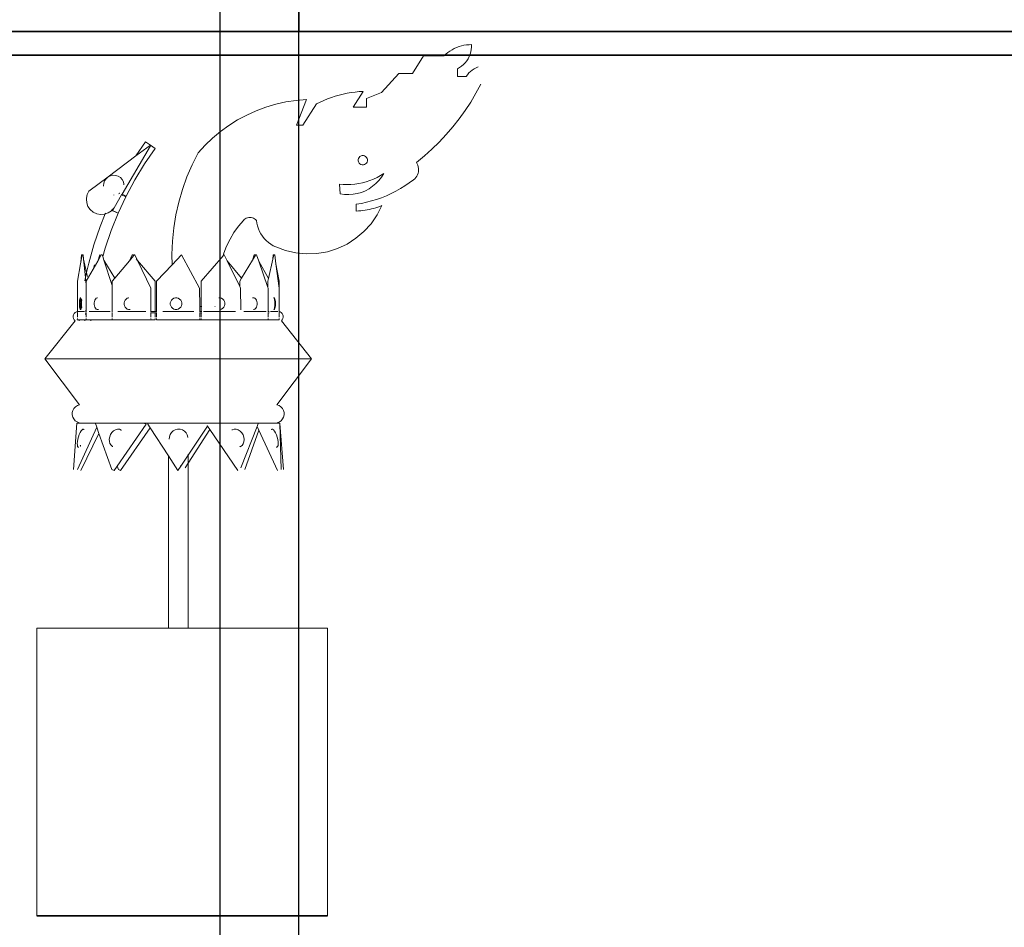
# Model space of a CAD drawing. Units: millimetres. Extents: x 446512 to 447461, y 70395 to 70610.
# Tile 3 of 39: x 446693.54 to 446714.29, y 70434.51 to 70453.63. Entities that reach past the tile are written whole.
import ezdxf

# ---------------------------------------------------------------- set-up
doc = ezdxf.new("R2010")
doc.units = ezdxf.units.MM
for name, color, linetype, lineweight in [('A-ANNO-DIMS', 2, 'Continuous', 18), ('A-FURN', 7, 'Continuous', 35), ('A-FURN-DECO', 8, 'Continuous', 13)]:
    doc.layers.add(name, color=color, linetype=linetype, lineweight=lineweight)
doc.styles.get("Standard").update_dxf_attribs({"font": 'arial.ttf'})
doc.dimstyles.get("Standard").update_dxf_attribs({"dimtxt": 0.18, "dimasz": 0.18, "dimexe": 0.18, "dimexo": 0.0625, "dimgap": 0.09, "dimtad": 0, "dimtih": 1, "dimtoh": 1, "dimdec": 4, "dimzin": 0, "dimdsep": 46, "dimtxsty": 'Standard', "dimcen": 0.09, "dimadec": 0, "dimazin": 0, "dimtfac": 1, "dimtdec": 4, "dimtofl": 0, "dimtmove": 0, "dimatfit": 3, "dimfxl": 1, "dimtolj": 1, "dimtzin": 0, "dimarcsym": 0})

# ---------------------------------------------------------------- blocks, each defined once
blk = doc.blocks.new('*D38')
at = {"layer": 'A-ANNO-DIMS', "color": 0, "lineweight": -2, "transparency": 16777216}
for p, q in [((446687.323552, 70428.838404), (446687.323552, 70578.17492)), ((446697.765686, 70428.838404), (446697.765686, 70578.17492)), ((446687.503552, 70577.99492), (446692.090383, 70577.99492)), ((446697.585686, 70577.99492), (446692.998855, 70577.99492))]:
    blk.add_line(p, q, dxfattribs=at)
at = {"layer": 'A-ANNO-DIMS', "color": 0, "transparency": 16777216}
for points in [[(446687.503552, 70578.02492), (446687.503552, 70577.96492), (446687.323552, 70577.99492)], [(446697.585686, 70578.02492), (446697.585686, 70577.96492), (446697.765686, 70577.99492)]]:
    blk.add_solid(points, dxfattribs=at)
at = {"layer": 'Defpoints', "color": 0, "transparency": 16777216}
for p in [(446697.765686, 70577.99492), (446687.323552, 70428.775904), (446697.765686, 70428.775904)]:
    blk.add_point(p, dxfattribs=at)
at = {"layer": 'A-ANNO-DIMS', "color": 0, "transparency": 16777216, "insert": (446692.544619, 70577.99492), "char_height": 0.18, "attachment_point": 5}
blk.add_mtext('\\A1;10.442', dxfattribs=at)
blk = doc.blocks.new('*D39')
at = {"layer": 'A-ANNO-DIMS', "color": 0, "lineweight": -2, "transparency": 16777216}
for p, q in [((446697.766, 70428.838), (446697.766, 70578.175)), ((446699.429, 70433.444), (446699.429, 70578.175)), ((446697.946, 70577.995), (446698.212, 70577.995)), ((446699.249, 70577.995), (446698.982, 70577.995))]:
    blk.add_line(p, q, dxfattribs=at)
at = {"layer": 'A-ANNO-DIMS', "color": 0, "transparency": 16777216}
for points in [[(446697.946, 70578.025), (446697.946, 70577.965), (446697.766, 70577.995)], [(446699.249, 70578.025), (446699.249, 70577.965), (446699.429, 70577.995)]]:
    blk.add_solid(points, dxfattribs=at)
at = {"layer": 'Defpoints', "color": 0, "transparency": 16777216}
for p in [(446699.429, 70577.995), (446699.429, 70433.382), (446697.766, 70428.776)]:
    blk.add_point(p, dxfattribs=at)
at = {"layer": 'A-ANNO-DIMS', "color": 0, "transparency": 16777216, "insert": (446698.597, 70577.995), "char_height": 0.18, "attachment_point": 5}
blk.add_mtext('\\A1;1.663', dxfattribs=at)

msp = doc.modelspace()

# ---------------------------------------------------------------- linework, layer by layer
at = {"layer": 'A-FURN'}
for p, q in [((446699.4288, 70473.3815), (446699.4288, 70453.3815)), ((446686.5728, 70453.3815), (446746.5728, 70453.3815)), ((446693.9059, 70434.754), (446700.0326, 70434.754))]:
    msp.add_line(p, q, dxfattribs=at)
for points in [[(446699.4288, 70473.3815), (446746.5728, 70473.3815), (446746.5728, 70453.3815), (446699.4288, 70453.3815)], [(446686.5728, 70453.3815), (446729.0084, 70453.3815), (446729.0084, 70433.3815), (446686.5728, 70433.3815)], [(446687.0728, 70452.8815), (446728.5084, 70452.8815), (446728.5084, 70433.8815), (446687.0728, 70433.8815)]]:
    msp.add_lwpolyline(points, close=True, dxfattribs=at)
at = {"layer": 'A-FURN-DECO'}
for p, q in [((446702.8542, 70453.0797), (446702.9068, 70453.0916)), ((446702.9068, 70453.0916), (446702.96, 70453.1001)), ((446702.96, 70453.1001), (446703.0136, 70453.1052)), ((446703.0136, 70453.1052), (446703.0675, 70453.1069)), ((446703.0675, 70453.1069), (446703.0671, 70453.0551)), ((446702.482, 70452.8715), (446702.522, 70452.9076)), ((446702.522, 70452.9076), (446702.5643, 70452.941)), ((446702.5643, 70452.941), (446702.6086, 70452.9717)), ((446702.6086, 70452.9717), (446702.6547, 70452.9995)), ((446702.6547, 70452.9995), (446702.7026, 70453.0243)), ((446702.7026, 70453.0243), (446702.7519, 70453.046)), ((446702.7519, 70453.046), (446702.8025, 70453.0645)), ((446702.8025, 70453.0645), (446702.8542, 70453.0797)), ((446703.0368, 70452.9034), (446703.0173, 70452.8555)), ((446703.0517, 70452.953), (446703.0368, 70452.9034)), ((446703.0618, 70453.0037), (446703.0517, 70452.953)), ((446703.0671, 70453.0551), (446703.0618, 70453.0037)), ((446701.8209, 70452.4964), (446702.0531, 70452.8715)), ((446702.0531, 70452.8715), (446702.482, 70452.8715)), ((446702.8973, 70452.6884), (446702.8581, 70452.6546)), ((446702.9331, 70452.7257), (446702.8973, 70452.6884)), ((446702.9652, 70452.7662), (446702.9331, 70452.7257)), ((446702.9934, 70452.8096), (446702.9652, 70452.7662)), ((446703.0173, 70452.8555), (446702.9934, 70452.8096)), ((446701.1687, 70452.0989), (446701.533, 70452.4964)), ((446701.533, 70452.4964), (446701.8209, 70452.4964)), ((446702.8159, 70452.6247), (446702.7711, 70452.5989)), ((446702.7711, 70452.5989), (446702.7711, 70452.4334)), ((446702.8581, 70452.6546), (446702.8159, 70452.6247)), ((446702.9549, 70452.4334), (446702.9812, 70452.4724)), ((446702.9812, 70452.4724), (446703.0111, 70452.5087)), ((446703.0111, 70452.5087), (446703.0443, 70452.5419)), ((446703.0443, 70452.5419), (446703.0806, 70452.5717)), ((446703.0806, 70452.5717), (446703.1197, 70452.5979)), ((446703.1197, 70452.5979), (446703.161, 70452.6202)), ((446703.161, 70452.6202), (446703.2044, 70452.6384)), ((446702.7711, 70452.4334), (446702.9549, 70452.4334)), ((446703.2601, 70452.271), (446703.1593, 70452.0812)), ((446700.2767, 70452.0427), (446700.3601, 70452.0633)), ((446700.3601, 70452.0633), (446700.4442, 70452.0808)), ((446700.4442, 70452.0808), (446700.5289, 70452.0954)), ((446700.5289, 70452.0954), (446700.614, 70452.1069)), ((446700.7853, 70452.1207), (446700.5738, 70451.7905)), ((446700.614, 70452.1069), (446700.6995, 70452.1153)), ((446700.6995, 70452.1153), (446700.7853, 70452.1207)), ((446700.8556, 70451.9743), (446701.1687, 70452.0989)), ((446703.1593, 70452.0812), (446703.0501, 70451.8961)), ((446698.732, 70451.7893), (446698.9413, 70451.8514)), ((446698.9413, 70451.8514), (446699.1544, 70451.8991)), ((446699.1544, 70451.8991), (446699.3702, 70451.9323)), ((446699.3702, 70451.9323), (446699.5878, 70451.9507)), ((446699.5878, 70451.9507), (446699.3741, 70451.4093)), ((446699.5089, 70451.4093), (446699.7964, 70451.8582)), ((446699.7964, 70451.8582), (446699.8735, 70451.896)), ((446699.8735, 70451.896), (446699.9519, 70451.9311)), ((446699.9519, 70451.9311), (446700.0316, 70451.9633)), ((446700.0316, 70451.9633), (446700.1123, 70451.9927)), ((446700.1123, 70451.9927), (446700.1941, 70452.0192)), ((446700.1941, 70452.0192), (446700.2767, 70452.0427)), ((446700.8556, 70451.7905), (446700.8556, 70451.9743)), ((446703.0501, 70451.8961), (446702.9328, 70451.716)), ((446698.3283, 70451.6233), (446698.5273, 70451.7132)), ((446698.5273, 70451.7132), (446698.732, 70451.7893)), ((446700.5738, 70451.7905), (446700.8556, 70451.7905)), ((446702.9328, 70451.716), (446702.8075, 70451.5413)), ((446697.9509, 70451.4041), (446698.1359, 70451.5201)), ((446698.1359, 70451.5201), (446698.3283, 70451.6233)), ((446702.8075, 70451.5413), (446702.6746, 70451.3724)), ((446697.6067, 70451.1358), (446697.7742, 70451.2758)), ((446697.7742, 70451.2758), (446697.9509, 70451.4041)), ((446699.3741, 70451.4093), (446699.5089, 70451.4093)), ((446702.6746, 70451.3724), (446702.5343, 70451.2096)), ((446696.1978, 70451.0593), (446695.9941, 70450.762)), ((446696.2989, 70450.9901), (446696.1978, 70451.0593)), ((446697.449, 70450.9847), (446697.6067, 70451.1358)), ((446702.3869, 70451.0532), (446702.2327, 70450.9035)), ((446702.5343, 70451.2096), (446702.3869, 70451.0532)), ((446696.2989, 70450.9742), (446695.7002, 70449.9534)), ((446696.2989, 70450.9901), (446695.9941, 70450.762)), ((446696.1758, 70450.5935), (446696.4, 70450.9208)), ((446696.2989, 70450.9742), (446696.2989, 70450.9901)), ((446696.4, 70450.9208), (446696.2989, 70450.9901)), ((446697.302, 70450.8233), (446697.1763, 70450.5748)), ((446697.302, 70450.8233), (446697.449, 70450.9847)), ((446702.2327, 70450.9035), (446702.0719, 70450.7609)), ((446695.9941, 70450.762), (446695.4048, 70450.3183)), ((446700.6765, 70450.6582), (446700.6767, 70450.6838)), ((446700.683, 70450.6335), (446700.6765, 70450.6582)), ((446700.6767, 70450.6838), (446700.6834, 70450.7085)), ((446700.6957, 70450.6113), (446700.683, 70450.6335)), ((446700.6834, 70450.7085), (446700.6963, 70450.7306)), ((446700.7137, 70450.5931), (446700.6957, 70450.6113)), ((446700.6963, 70450.7306), (446700.7145, 70450.7486)), ((446700.7145, 70450.7486), (446700.7368, 70450.7613)), ((446700.7368, 70450.7613), (446700.7615, 70450.7678)), ((446700.7615, 70450.7678), (446700.7871, 70450.7677)), ((446700.7871, 70450.7677), (446700.8118, 70450.7609)), ((446700.8118, 70450.7609), (446700.8339, 70450.748)), ((446700.8513, 70450.6105), (446700.8331, 70450.5925)), ((446700.8339, 70450.748), (446700.8519, 70450.7298)), ((446700.8642, 70450.6326), (446700.8513, 70450.6105)), ((446700.8519, 70450.7298), (446700.8646, 70450.7076)), ((446700.8709, 70450.6572), (446700.8642, 70450.6326)), ((446700.8646, 70450.7076), (446700.8711, 70450.6828)), ((446700.8711, 70450.6828), (446700.8709, 70450.6572)), ((446702.0719, 70450.7609), (446701.9049, 70450.6255)), ((446701.9049, 70450.6255), (446701.922, 70450.5959)), ((446695.9713, 70450.2574), (446696.1758, 70450.5935)), ((446697.1763, 70450.5748), (446697.0663, 70450.3191)), ((446700.7358, 70450.5802), (446700.7137, 70450.5931)), ((446700.7605, 70450.5734), (446700.7358, 70450.5802)), ((446700.7861, 70450.5733), (446700.7605, 70450.5734)), ((446700.8108, 70450.5798), (446700.7861, 70450.5733)), ((446700.8331, 70450.5925), (446700.8108, 70450.5798)), ((446701.2148, 70450.393), (446701.1455, 70450.3494)), ((446701.2148, 70450.393), (446701.1676, 70450.3162)), ((446701.922, 70450.5959), (446701.9352, 70450.5643)), ((446701.9389, 70450.3958), (446701.9271, 70450.3636)), ((446701.9352, 70450.5643), (446701.9444, 70450.5313)), ((446701.9467, 70450.4291), (446701.9389, 70450.3958)), ((446701.9444, 70450.5313), (446701.9494, 70450.4974)), ((446701.9502, 70450.4632), (446701.9467, 70450.4291)), ((446701.9494, 70450.4974), (446701.9502, 70450.4632)), ((446695.4048, 70450.3183), (446695.0009, 70450.0187)), ((446695.3124, 70450.1313), (446695.3153, 70450.1853)), ((446695.3153, 70450.1853), (446695.3327, 70450.2368)), ((446695.3327, 70450.2368), (446695.3632, 70450.2821)), ((446695.3632, 70450.2821), (446695.4048, 70450.3183)), ((446695.4048, 70450.3183), (446695.4547, 70450.3428)), ((446695.4547, 70450.3428), (446695.5094, 70450.354)), ((446695.5094, 70450.354), (446695.5653, 70450.3512)), ((446695.5653, 70450.3512), (446695.6185, 70450.3344)), ((446695.6185, 70450.3344), (446695.6655, 70450.305)), ((446695.6655, 70450.305), (446695.7029, 70450.2648)), ((446695.7029, 70450.2648), (446695.7283, 70450.2166)), ((446695.7283, 70450.2166), (446695.74, 70450.1637)), ((446695.9713, 70450.2574), (446695.7853, 70449.9107)), ((446697.0663, 70450.3191), (446696.9722, 70450.057)), ((446700.7676, 70450.1961), (446700.6876, 70450.1792)), ((446700.8465, 70450.2178), (446700.7676, 70450.1961)), ((446700.9241, 70450.244), (446700.8465, 70450.2178)), ((446700.9999, 70450.2748), (446700.9241, 70450.244)), ((446701.0738, 70450.3099), (446700.9999, 70450.2748)), ((446701.1126, 70450.2448), (446701.0504, 70450.1797)), ((446701.1455, 70450.3494), (446701.0738, 70450.3099)), ((446701.1676, 70450.3162), (446701.1126, 70450.2448)), ((446701.7545, 70450.1914), (446701.6629, 70450.1297)), ((446701.8434, 70450.2569), (446701.7545, 70450.1914)), ((446701.8692, 70450.2794), (446701.8434, 70450.2569)), ((446701.8919, 70450.305), (446701.8692, 70450.2794)), ((446701.9114, 70450.3332), (446701.8919, 70450.305)), ((446701.9271, 70450.3636), (446701.9114, 70450.3332)), ((446695.0009, 70450.0187), (446694.9648, 70449.9466)), ((446695.3128, 70450.1294), (446695.3124, 70450.1313)), ((446695.3124, 70450.1218), (446695.3128, 70450.1294)), ((446695.6567, 70449.9752), (446695.6498, 70449.9787)), ((446695.7395, 70450.1561), (446695.74, 70450.1637)), ((446695.7395, 70450.1561), (446695.74, 70450.1542)), ((446696.9722, 70450.057), (446696.8945, 70449.7897)), ((446700.3616, 70450.159), (446700.28, 70450.166)), ((446700.28, 70450.166), (446700.3001, 70449.9625)), ((446700.4434, 70450.1569), (446700.3616, 70450.159)), ((446700.5252, 70450.1595), (446700.4434, 70450.1569)), ((446700.6066, 70450.167), (446700.5252, 70450.1595)), ((446700.6876, 70450.1792), (446700.6066, 70450.167)), ((446700.7444, 70449.994), (446700.6579, 70449.969)), ((446700.8279, 70450.028), (446700.7444, 70449.994)), ((446700.9072, 70450.0707), (446700.8279, 70450.028)), ((446700.9817, 70450.1214), (446700.9072, 70450.0707)), ((446701.0504, 70450.1797), (446700.9817, 70450.1214)), ((446701.4724, 70450.0182), (446701.3738, 70449.9685)), ((446701.5688, 70450.072), (446701.4724, 70450.0182)), ((446701.6629, 70450.1297), (446701.5688, 70450.072)), ((446694.9648, 70449.9466), (446694.9494, 70449.868)), ((446694.9494, 70449.8521), (446694.9494, 70449.868)), ((446694.9494, 70449.8521), (446694.9555, 70449.7723)), ((446694.9555, 70449.7723), (446694.9828, 70449.6967)), ((446695.5291, 70449.9417), (446695.5248, 70449.9324)), ((446695.6917, 70449.9388), (446695.5318, 70449.6663)), ((446695.6194, 70449.5569), (446695.7792, 70449.8978)), ((446695.6296, 70449.9679), (446695.6395, 70449.9633)), ((446695.7002, 70449.9534), (446695.6917, 70449.9388)), ((446695.7792, 70449.8978), (446695.6917, 70449.9388)), ((446695.7002, 70449.9534), (446695.7853, 70449.9107)), ((446696.8945, 70449.7897), (446696.8335, 70449.518)), ((446700.3893, 70449.9499), (446700.3001, 70449.9625)), ((446700.4793, 70449.9468), (446700.3893, 70449.9499)), ((446700.5692, 70449.9532), (446700.4793, 70449.9468)), ((446700.6579, 70449.969), (446700.5692, 70449.9532)), ((446700.8544, 70449.7841), (446700.7466, 70449.7606)), ((446700.9612, 70449.8122), (446700.8544, 70449.7841)), ((446701.0667, 70449.8448), (446700.9612, 70449.8122)), ((446701.1708, 70449.8817), (446701.0667, 70449.8448)), ((446701.2732, 70449.9229), (446701.1708, 70449.8817)), ((446701.3738, 70449.9685), (446701.2732, 70449.9229)), ((446694.9828, 70449.6967), (446695.0294, 70449.6305)), ((446695.0294, 70449.6305), (446695.0922, 70449.5782)), ((446695.0922, 70449.5782), (446695.1668, 70449.5434)), ((446695.4092, 70449.5607), (446695.4777, 70449.6057)), ((446695.4724, 70449.6181), (446695.4842, 70449.6129)), ((446695.4777, 70449.6057), (446695.4842, 70449.6129)), ((446695.4888, 70449.6181), (446695.4797, 70449.6224)), ((446695.4842, 70449.6129), (446695.4888, 70449.6181)), ((446695.4842, 70449.6129), (446695.6182, 70449.5545)), ((446695.4888, 70449.6181), (446695.5318, 70449.6663)), ((446695.4888, 70449.6181), (446695.6194, 70449.5569)), ((446695.5084, 70449.6089), (446695.5059, 70449.6035)), ((446695.5494, 70449.6962), (446695.5084, 70449.6089)), ((446700.7466, 70449.7606), (446700.6378, 70449.7416)), ((446700.6378, 70449.7416), (446700.6378, 70449.6006)), ((446700.6378, 70449.6006), (446700.6839, 70449.6028)), ((446700.6839, 70449.6028), (446700.73, 70449.6063)), ((446700.73, 70449.6063), (446700.7759, 70449.6112)), ((446700.7759, 70449.6112), (446700.8217, 70449.6174)), ((446700.8217, 70449.6174), (446700.8673, 70449.625)), ((446700.8673, 70449.625), (446700.9126, 70449.6339)), ((446700.9126, 70449.6339), (446700.9576, 70449.6441)), ((446700.9576, 70449.6441), (446701.0023, 70449.6557)), ((446701.0023, 70449.6557), (446701.0467, 70449.6686)), ((446701.0467, 70449.6686), (446701.0907, 70449.6828)), ((446701.1772, 70449.715), (446701.0758, 70449.5169)), ((446701.0907, 70449.6828), (446701.1342, 70449.6983)), ((446701.1342, 70449.6983), (446701.1772, 70449.715)), ((446695.1668, 70449.5434), (446695.2482, 70449.5284)), ((446695.3481, 70449.5401), (446695.2411, 70449.2755)), ((446695.2482, 70449.5284), (446695.3309, 70449.5343)), ((446695.3309, 70449.5343), (446695.3481, 70449.5401)), ((446695.3481, 70449.5401), (446695.4092, 70449.5607)), ((446695.3555, 70449.5584), (446695.3481, 70449.5401)), ((446695.4707, 70449.1897), (446695.6182, 70449.5545)), ((446696.8335, 70449.518), (446696.7894, 70449.2431)), ((446698.2574, 70449.4038), (446698.1536, 70449.2792)), ((446698.276, 70449.4217), (446698.2574, 70449.4038)), ((446698.297, 70449.4369), (446698.276, 70449.4217)), ((446698.3198, 70449.449), (446698.297, 70449.4369)), ((446698.3442, 70449.4579), (446698.3198, 70449.449)), ((446698.3695, 70449.4632), (446698.3442, 70449.4579)), ((446698.3953, 70449.465), (446698.3695, 70449.4632)), ((446698.4211, 70449.4632), (446698.3953, 70449.465)), ((446698.4464, 70449.4579), (446698.4211, 70449.4632)), ((446698.4707, 70449.449), (446698.4464, 70449.4579)), ((446698.4935, 70449.4369), (446698.4707, 70449.449)), ((446698.5145, 70449.4217), (446698.4935, 70449.4369)), ((446698.5331, 70449.4038), (446698.5145, 70449.4217)), ((446698.542, 70449.344), (446698.5331, 70449.4038)), ((446701.0758, 70449.5169), (446700.9493, 70449.3338)), ((446695.2411, 70449.2755), (446695.1092, 70448.8908)), ((446695.3431, 70448.8176), (446695.4707, 70449.1897)), ((446696.7894, 70449.2431), (446696.7623, 70448.966)), ((446698.1536, 70449.2792), (446698.0599, 70449.1468)), ((446698.5561, 70449.2853), (446698.542, 70449.344)), ((446698.5752, 70449.228), (446698.5561, 70449.2853)), ((446698.5992, 70449.1726), (446698.5752, 70449.228)), ((446698.628, 70449.1195), (446698.5992, 70449.1726)), ((446700.7997, 70449.169), (446700.6297, 70449.0253)), ((446700.9493, 70449.3338), (446700.7997, 70449.169)), ((446696.7623, 70448.966), (446696.7524, 70448.6878)), ((446697.9769, 70449.0074), (446697.9052, 70448.8619)), ((446698.0599, 70449.1468), (446697.9769, 70449.0074)), ((446698.6613, 70449.0692), (446698.628, 70449.1195)), ((446698.6988, 70449.0218), (446698.6613, 70449.0692)), ((446698.7403, 70448.978), (446698.6988, 70449.0218)), ((446698.7855, 70448.9379), (446698.7403, 70448.978)), ((446700.6297, 70449.0253), (446700.4423, 70448.9053)), ((446695.1092, 70448.8908), (446694.9983, 70448.4995)), ((446695.2935, 70448.6424), (446695.3431, 70448.8176)), ((446697.9052, 70448.8619), (446697.8452, 70448.7113)), ((446698.834, 70448.9019), (446698.7855, 70448.9379)), ((446698.8854, 70448.8702), (446698.834, 70448.9019)), ((446698.9394, 70448.8432), (446698.8854, 70448.8702)), ((446699.1481, 70448.7658), (446698.9394, 70448.8432)), ((446699.3651, 70448.7166), (446699.1481, 70448.7658)), ((446700.0284, 70448.7441), (446699.8092, 70448.7057)), ((446700.2407, 70448.811), (446700.0284, 70448.7441)), ((446700.4423, 70448.9053), (446700.2407, 70448.811)), ((446694.8288, 70448.5236), (446694.8482, 70448.6763)), ((446694.8582, 70448.6763), (446694.8288, 70448.5236)), ((446694.8582, 70448.6763), (446694.8482, 70448.6763)), ((446694.8582, 70448.6763), (446694.8822, 70448.6763)), ((446694.8913, 70448.5887), (446694.8822, 70448.6763)), ((446694.8913, 70448.5887), (446694.9539, 70448.3032)), ((446694.9313, 70448.203), (446694.8913, 70448.5887)), ((446695.1878, 70448.5442), (446694.9473, 70448.1202)), ((446695.1878, 70448.5442), (446695.2337, 70448.6763)), ((446695.2627, 70448.6763), (446695.1878, 70448.5442)), ((446695.2394, 70448.6763), (446695.2337, 70448.6763)), ((446695.2824, 70448.6763), (446695.2627, 70448.6763)), ((446695.2935, 70448.6424), (446695.2824, 70448.6763)), ((446695.3183, 70448.5668), (446695.2935, 70448.6424)), ((446695.3183, 70448.5668), (446695.5476, 70448.1845)), ((446695.4941, 70448.0319), (446695.3183, 70448.5668)), ((446695.8544, 70448.5528), (446695.5476, 70448.1845)), ((446695.8544, 70448.5528), (446695.9153, 70448.6763)), ((446695.9418, 70448.6578), (446695.8544, 70448.5528)), ((446695.926, 70448.6763), (446695.9153, 70448.6763)), ((446695.926, 70448.6763), (446695.9418, 70448.6578)), ((446695.9572, 70448.6763), (446695.9418, 70448.6578)), ((446695.9689, 70448.6763), (446695.9572, 70448.6763)), ((446696.0249, 70448.5602), (446695.9689, 70448.6763)), ((446695.998, 70448.5918), (446696.0249, 70448.5602)), ((446696.0249, 70448.5602), (446696.3997, 70448.1202)), ((446696.3058, 70447.978), (446696.0249, 70448.5602)), ((446696.7524, 70448.6878), (446696.7582, 70448.4702)), ((446696.9532, 70448.6763), (446696.7582, 70448.4702)), ((446697.3363, 70447.978), (446696.9532, 70448.6763)), ((446697.8282, 70448.6563), (446697.3691, 70448.1202)), ((446697.8282, 70448.6563), (446697.8235, 70448.6412)), ((446697.8296, 70448.6609), (446697.8282, 70448.6563)), ((446697.8282, 70448.6563), (446697.8323, 70448.6514)), ((446697.8452, 70448.7113), (446697.8296, 70448.6609)), ((446697.8427, 70448.6763), (446697.8296, 70448.6609)), ((446697.8427, 70448.6763), (446697.8534, 70448.6763)), ((446697.9144, 70448.5528), (446697.8534, 70448.6763)), ((446697.9144, 70448.5528), (446698.2211, 70448.1845)), ((446697.9144, 70448.5528), (446698.1826, 70448.0092)), ((446698.4504, 70448.5668), (446698.2211, 70448.1845)), ((446698.4504, 70448.5668), (446698.4864, 70448.6763)), ((446698.5109, 70448.6677), (446698.4504, 70448.5668)), ((446698.4864, 70448.6763), (446698.506, 70448.6763)), ((446698.506, 70448.6763), (446698.5109, 70448.6677)), ((446698.5161, 70448.6763), (446698.5109, 70448.6677)), ((446698.5161, 70448.6763), (446698.535, 70448.6763)), ((446698.5809, 70448.5442), (446698.535, 70448.6763)), ((446698.5809, 70448.5442), (446698.7877, 70448.1796)), ((446698.5809, 70448.5442), (446698.7747, 70447.9866)), ((446698.8775, 70448.5887), (446698.7877, 70448.1796)), ((446698.8775, 70448.5887), (446698.8865, 70448.6763)), ((446698.8967, 70448.6763), (446698.8775, 70448.5887)), ((446698.8865, 70448.6763), (446698.8967, 70448.6763)), ((446698.8967, 70448.6763), (446698.9205, 70448.6763)), ((446698.9205, 70448.6763), (446698.9448, 70448.4854)), ((446699.5868, 70448.6965), (446699.3651, 70448.7166)), ((446699.8092, 70448.7057), (446699.5868, 70448.6965)), ((446694.824, 70448.4854), (446694.7586, 70448.1202)), ((446694.824, 70448.4854), (446694.8288, 70448.5236)), ((446694.9983, 70448.4995), (446694.9539, 70448.3032)), ((446695.1171, 70448.4693), (446695.0983, 70448.3864)), ((446696.7582, 70448.4702), (446696.4267, 70448.1202)), ((446698.9448, 70448.4854), (446699.0102, 70448.1202)), ((446699.0093, 70447.978), (446698.9448, 70448.4854)), ((446694.7586, 70448.1202), (446694.7606, 70447.9867)), ((446694.9313, 70448.203), (446694.9148, 70448.13)), ((446694.9539, 70448.3032), (446694.9313, 70448.203)), ((446694.9473, 70448.0484), (446694.9313, 70448.203)), ((446694.9473, 70448.1202), (446694.9473, 70448.0484)), ((446694.9539, 70448.3032), (446694.9721, 70448.2206)), ((446695.5476, 70448.1845), (446695.4941, 70448.1202)), ((446695.4941, 70448.1202), (446695.4941, 70448.0319)), ((446696.3997, 70448.1202), (446696.3997, 70447.4807)), ((446696.4267, 70448.1202), (446696.4267, 70447.4807)), ((446697.3691, 70448.1202), (446697.3691, 70447.5888)), ((446698.2211, 70448.1845), (446698.1826, 70448.1202)), ((446698.1826, 70448.1202), (446698.1826, 70448.0092)), ((446698.7877, 70448.1796), (446698.7747, 70448.1202)), ((446698.7747, 70448.1202), (446698.7747, 70447.9866)), ((446699.0102, 70448.1202), (446699.0093, 70447.978)), ((446694.7595, 70447.978), (446694.7585, 70447.4791)), ((446694.7595, 70447.978), (446694.7606, 70447.9867)), ((446694.9473, 70448.0484), (446694.9473, 70447.4807)), ((446695.4941, 70448.0319), (446695.4941, 70447.4739)), ((446696.3058, 70447.978), (446696.3096, 70447.4807)), ((446697.3363, 70447.978), (446697.3396, 70447.5885)), ((446698.198, 70447.978), (446698.1826, 70448.0092)), ((446698.198, 70447.978), (446698.2016, 70447.5183)), ((446698.7776, 70447.978), (446698.7747, 70447.9866)), ((446698.7776, 70447.978), (446698.7804, 70447.4807)), ((446699.0093, 70447.978), (446699.0103, 70447.4791)), ((446694.8017, 70447.6648), (446694.8032, 70447.6957)), ((446694.8032, 70447.6957), (446694.8063, 70447.7234)), ((446694.8063, 70447.7234), (446694.8106, 70447.7459)), ((446694.8106, 70447.7459), (446694.8158, 70447.7619)), ((446694.8137, 70447.6648), (446694.8153, 70447.6957)), ((446694.8153, 70447.6957), (446694.8183, 70447.7234)), ((446694.8158, 70447.7619), (446694.8217, 70447.7701)), ((446694.8183, 70447.7234), (446694.8226, 70447.7459)), ((446694.8337, 70447.7701), (446694.8217, 70447.7701)), ((446694.8226, 70447.7459), (446694.8279, 70447.7619)), ((446694.8279, 70447.7619), (446694.8337, 70447.7701)), ((446694.8364, 70447.6951), (446694.8345, 70447.6642)), ((446694.8401, 70447.7229), (446694.8364, 70447.6951)), ((446694.8406, 70447.7018), (446694.8364, 70447.6951)), ((446694.8453, 70447.7455), (446694.8401, 70447.7229)), ((446694.8401, 70447.7229), (446694.8406, 70447.7018)), ((446694.8483, 70447.7531), (446694.8453, 70447.7455)), ((446694.849, 70447.7511), (446694.8453, 70447.7455)), ((446694.8483, 70447.6951), (446694.8464, 70447.6642)), ((446694.852, 70447.7229), (446694.8483, 70447.6951)), ((446694.8537, 70447.7302), (446694.852, 70447.7229)), ((446695.1121, 70447.6648), (446695.1171, 70447.6957)), ((446695.1171, 70447.6957), (446695.1267, 70447.7234)), ((446695.1267, 70447.7234), (446695.1403, 70447.7459)), ((446695.1403, 70447.7459), (446695.1569, 70447.7619)), ((446695.1569, 70447.7619), (446695.1755, 70447.7701)), ((446695.1853, 70447.7701), (446695.1755, 70447.7701)), ((446695.7446, 70447.6648), (446695.7519, 70447.6957)), ((446695.7519, 70447.6957), (446695.7661, 70447.7234)), ((446695.7661, 70447.7234), (446695.786, 70447.7459)), ((446695.786, 70447.7459), (446695.8104, 70447.7619)), ((446695.8104, 70447.7619), (446695.8376, 70447.7701)), ((446695.8435, 70447.7701), (446695.8376, 70447.7701)), ((446696.7182, 70447.6648), (446696.7265, 70447.6957)), ((446696.7265, 70447.6957), (446696.7426, 70447.7234)), ((446696.7426, 70447.7234), (446696.7653, 70447.7459)), ((446696.7653, 70447.7459), (446696.793, 70447.7619)), ((446696.793, 70447.7619), (446696.8239, 70447.7701)), ((446696.8239, 70447.7701), (446696.8559, 70447.77)), ((446696.8559, 70447.77), (446696.8868, 70447.7616)), ((446696.8868, 70447.7616), (446696.9144, 70447.7455)), ((446696.9144, 70447.7455), (446696.937, 70447.7229)), ((446696.937, 70447.7229), (446696.9529, 70447.6951)), ((446696.9529, 70447.6951), (446696.9611, 70447.6642)), ((446697.7371, 70447.7701), (446697.7425, 70447.7701)), ((446697.7425, 70447.7701), (446697.7712, 70447.77)), ((446697.7712, 70447.77), (446697.799, 70447.7616)), ((446697.799, 70447.7616), (446697.8239, 70447.7455)), ((446697.8239, 70447.7455), (446697.8442, 70447.7229)), ((446697.8442, 70447.7229), (446697.8585, 70447.6951)), ((446697.8585, 70447.6951), (446697.8659, 70447.6642)), ((446698.4531, 70447.7701), (446698.4626, 70447.7701)), ((446698.4626, 70447.7701), (446698.4829, 70447.77)), ((446698.4829, 70447.77), (446698.5024, 70447.7616)), ((446698.5024, 70447.7616), (446698.52, 70447.7455)), ((446698.52, 70447.7455), (446698.5342, 70447.7229)), ((446698.5342, 70447.7229), (446698.5443, 70447.6951)), ((446698.5443, 70447.6951), (446698.5495, 70447.6642)), ((446698.8906, 70447.7701), (446698.898, 70447.77)), ((446698.898, 70447.77), (446698.9025, 70447.7701)), ((446698.898, 70447.77), (446698.9051, 70447.7616)), ((446698.9025, 70447.7701), (446698.9099, 70447.77)), ((446698.9051, 70447.7616), (446698.9115, 70447.7455)), ((446698.9099, 70447.77), (446698.917, 70447.7616)), ((446698.9115, 70447.7455), (446698.9168, 70447.7229)), ((446698.9168, 70447.7229), (446698.9204, 70447.6951)), ((446698.917, 70447.7616), (446698.9235, 70447.7455)), ((446698.9204, 70447.6951), (446698.9223, 70447.6642)), ((446698.9235, 70447.7455), (446698.9287, 70447.7229)), ((446698.9287, 70447.7229), (446698.9324, 70447.6951)), ((446698.9324, 70447.6951), (446698.9343, 70447.6642)), ((446694.8016, 70447.6329), (446694.8017, 70447.6648)), ((446694.8032, 70447.6019), (446694.8016, 70447.6329)), ((446694.8062, 70447.5742), (446694.8032, 70447.6019)), ((446694.8105, 70447.5515), (446694.8062, 70447.5742)), ((446694.8157, 70447.5354), (446694.8105, 70447.5515)), ((446694.8137, 70447.6329), (446694.8137, 70447.6648)), ((446694.8152, 70447.6019), (446694.8137, 70447.6329)), ((446694.8182, 70447.5742), (446694.8152, 70447.6019)), ((446694.8215, 70447.5271), (446694.8157, 70447.5354)), ((446694.8225, 70447.5515), (446694.8182, 70447.5742)), ((446694.8276, 70447.527), (446694.8215, 70447.5271)), ((446694.8345, 70447.6322), (446694.8225, 70447.5515)), ((446694.8277, 70447.5354), (446694.8225, 70447.5515)), ((446694.8336, 70447.5271), (446694.8276, 70447.527)), ((446694.8336, 70447.5271), (446694.8277, 70447.5354)), ((446694.8396, 70447.527), (446694.8336, 70447.5271)), ((446694.8345, 70447.6642), (446694.8345, 70447.6322)), ((446694.8345, 70447.6322), (446694.8365, 70447.6013)), ((446694.8365, 70447.6013), (446694.8402, 70447.5737)), ((446694.8402, 70447.5737), (446694.8454, 70447.5511)), ((446694.8454, 70447.5511), (446694.8483, 70447.5439)), ((446694.8464, 70447.6642), (446694.8464, 70447.6322)), ((446694.8464, 70447.6322), (446694.8484, 70447.6013)), ((446694.8484, 70447.6013), (446694.8521, 70447.5737)), ((446694.8521, 70447.5737), (446694.8537, 70447.5668)), ((446694.9473, 70447.5567), (446694.9379, 70447.4739)), ((446695.112, 70447.6329), (446695.1121, 70447.6648)), ((446695.117, 70447.6019), (446695.112, 70447.6329)), ((446695.1265, 70447.5742), (446695.117, 70447.6019)), ((446695.14, 70447.5515), (446695.1265, 70447.5742)), ((446695.1566, 70447.5354), (446695.14, 70447.5515)), ((446695.1751, 70447.5271), (446695.1566, 70447.5354)), ((446695.1942, 70447.527), (446695.1751, 70447.5271)), ((446695.204, 70447.527), (446695.1942, 70447.527)), ((446695.7445, 70447.6329), (446695.7446, 70447.6648)), ((446695.7517, 70447.6019), (446695.7445, 70447.6329)), ((446695.7657, 70447.5742), (446695.7517, 70447.6019)), ((446695.7856, 70447.5515), (446695.7657, 70447.5742)), ((446695.8099, 70447.5354), (446695.7856, 70447.5515)), ((446695.8371, 70447.5271), (446695.8099, 70447.5354)), ((446695.8652, 70447.527), (446695.8371, 70447.5271)), ((446695.871, 70447.527), (446695.8652, 70447.527)), ((446696.7181, 70447.6329), (446696.7182, 70447.6648)), ((446696.7263, 70447.6019), (446696.7181, 70447.6329)), ((446696.7422, 70447.5742), (446696.7263, 70447.6019)), ((446696.7647, 70447.5515), (446696.7422, 70447.5742)), ((446696.7924, 70447.5354), (446696.7647, 70447.5515)), ((446696.8233, 70447.5271), (446696.7924, 70447.5354)), ((446696.8553, 70447.527), (446696.8233, 70447.5271)), ((446696.8862, 70447.5352), (446696.8553, 70447.527)), ((446696.9139, 70447.5511), (446696.8862, 70447.5352)), ((446696.9366, 70447.5737), (446696.9139, 70447.5511)), ((446696.9527, 70447.6013), (446696.9366, 70447.5737)), ((446696.961, 70447.6322), (446696.9527, 70447.6013)), ((446696.9611, 70447.6642), (446696.961, 70447.6322)), ((446697.3691, 70447.5888), (446697.3396, 70447.5885)), ((446697.3396, 70447.5885), (446697.3406, 70447.4807)), ((446697.3798, 70447.5889), (446697.3691, 70447.5888)), ((446697.3691, 70447.5888), (446697.3691, 70447.4807)), ((446697.6601, 70447.5913), (446697.6548, 70447.5912)), ((446697.7653, 70447.527), (446697.7707, 70447.527)), ((446697.7985, 70447.5352), (446697.7707, 70447.527)), ((446697.8234, 70447.5511), (446697.7985, 70447.5352)), ((446697.8438, 70447.5737), (446697.8234, 70447.5511)), ((446697.8583, 70447.6013), (446697.8438, 70447.5737)), ((446697.8658, 70447.6322), (446697.8583, 70447.6013)), ((446697.8659, 70447.6642), (446697.8658, 70447.6322)), ((446698.473, 70447.527), (446698.4825, 70447.527)), ((446698.5021, 70447.5352), (446698.4825, 70447.527)), ((446698.5196, 70447.5511), (446698.5021, 70447.5352)), ((446698.534, 70447.5737), (446698.5196, 70447.5511)), ((446698.5442, 70447.6013), (446698.534, 70447.5737)), ((446698.5495, 70447.6322), (446698.5442, 70447.6013)), ((446698.5495, 70447.6642), (446698.5495, 70447.6322)), ((446698.905, 70447.5352), (446698.8978, 70447.527)), ((446698.8978, 70447.527), (446698.9097, 70447.527)), ((446698.9114, 70447.5511), (446698.905, 70447.5352)), ((446698.9169, 70447.5352), (446698.9097, 70447.527)), ((446698.9167, 70447.5737), (446698.9114, 70447.5511)), ((446698.9204, 70447.6013), (446698.9167, 70447.5737)), ((446698.9233, 70447.5511), (446698.9169, 70447.5352)), ((446698.9223, 70447.6322), (446698.9204, 70447.6013)), ((446698.9223, 70447.6642), (446698.9223, 70447.6322)), ((446698.9286, 70447.5737), (446698.9233, 70447.5511)), ((446698.9323, 70447.6013), (446698.9286, 70447.5737)), ((446698.9342, 70447.6322), (446698.9323, 70447.6013)), ((446698.9343, 70447.6642), (446698.9342, 70447.6322)), ((446694.0764, 70446.4874), (446694.7108, 70447.2901)), ((446694.6708, 70447.3618), (446694.6712, 70447.3897)), ((446694.6776, 70447.3346), (446694.6708, 70447.3618)), ((446694.6712, 70447.3897), (446694.6788, 70447.4167)), ((446694.6913, 70447.3102), (446694.6776, 70447.3346)), ((446694.6788, 70447.4167), (446694.6931, 70447.4407)), ((446694.7108, 70447.2901), (446694.6913, 70447.3102)), ((446694.6931, 70447.4407), (446694.7132, 70447.4602)), ((446694.7132, 70447.4602), (446694.7376, 70447.4739)), ((446694.7376, 70447.4739), (446694.7585, 70447.4791)), ((446694.7582, 70447.3346), (446694.7581, 70447.3102)), ((446694.7606, 70447.3102), (446694.7581, 70447.3102)), ((446694.7958, 70447.3102), (446694.7581, 70447.3102)), ((446694.7584, 70447.4602), (446694.7582, 70447.3618)), ((446694.7585, 70447.4791), (446694.7648, 70447.4807)), ((446694.7585, 70447.4791), (446694.7585, 70447.4739)), ((446694.7648, 70447.4807), (446694.7695, 70447.4806)), ((446694.7648, 70447.4807), (446694.7667, 70447.4807)), ((446694.9083, 70447.4807), (446694.7695, 70447.4806)), ((446694.7944, 70447.2978), (446694.7939, 70447.2901)), ((446694.7958, 70447.3102), (446694.7944, 70447.2978)), ((446694.9473, 70447.3102), (446694.7958, 70447.3102)), ((446694.9191, 70447.3102), (446694.9168, 70447.2901)), ((446694.9473, 70447.4807), (446694.9314, 70447.4807)), ((446694.9473, 70447.4583), (446694.9314, 70447.4583)), ((446694.9363, 70447.4602), (446694.9315, 70447.4183)), ((446694.9473, 70447.4807), (446694.9473, 70447.4739)), ((446694.9473, 70447.4602), (446694.9473, 70447.4583)), ((446694.9473, 70447.4583), (446694.9473, 70447.3618)), ((446694.9473, 70447.3346), (446694.9473, 70447.3102)), ((446694.9473, 70447.3102), (446695.0424, 70447.3102)), ((446695.4478, 70447.4807), (446695.0054, 70447.4807)), ((446695.0401, 70447.2901), (446695.0424, 70447.3102)), ((446695.0424, 70447.3102), (446695.4956, 70447.3102)), ((446695.4941, 70447.4602), (446695.4941, 70447.3618)), ((446695.4941, 70447.3346), (446695.4956, 70447.3102)), ((446695.4956, 70447.3102), (446696.3109, 70447.3102)), ((446695.6136, 70447.4807), (446696.2027, 70447.4807)), ((446696.3096, 70447.4807), (446696.2979, 70447.4807)), ((446696.3097, 70447.4583), (446696.2981, 70447.4583)), ((446696.3096, 70447.4807), (446696.3096, 70447.4739)), ((446696.3997, 70447.4807), (446696.3096, 70447.4807)), ((446696.3097, 70447.4602), (446696.3097, 70447.4583)), ((446696.3097, 70447.4583), (446696.3105, 70447.3618)), ((446696.3997, 70447.4583), (446696.3097, 70447.4583)), ((446696.3107, 70447.3346), (446696.3109, 70447.3102)), ((446696.3997, 70447.3102), (446696.3109, 70447.3102)), ((446696.3997, 70447.4807), (446696.4267, 70447.4807)), ((446696.3997, 70447.4807), (446696.3997, 70447.4739)), ((446696.3997, 70447.4602), (446696.3997, 70447.4583)), ((446696.3997, 70447.4583), (446696.3997, 70447.3618)), ((446696.4267, 70447.4583), (446696.3997, 70447.4583)), ((446696.3997, 70447.3346), (446696.3997, 70447.3102)), ((446696.4267, 70447.4807), (446696.4267, 70447.4739)), ((446696.4267, 70447.4602), (446696.4267, 70447.4583)), ((446696.4267, 70447.4583), (446696.4267, 70447.3618)), ((446696.4267, 70447.3346), (446696.4267, 70447.3102)), ((446696.4267, 70447.3102), (446697.342, 70447.3102)), ((446696.5586, 70447.4807), (446697.2102, 70447.4807)), ((446697.3406, 70447.4807), (446697.3406, 70447.4739)), ((446697.3691, 70447.4807), (446697.3406, 70447.4807)), ((446697.3407, 70447.4602), (446697.3408, 70447.4583)), ((446697.3408, 70447.4583), (446697.3416, 70447.3618)), ((446697.3691, 70447.4583), (446697.3408, 70447.4583)), ((446697.3418, 70447.3346), (446697.342, 70447.3102)), ((446697.3691, 70447.3102), (446697.342, 70447.3102)), ((446697.3798, 70447.4807), (446697.3691, 70447.4807)), ((446697.3691, 70447.4807), (446697.3691, 70447.4739)), ((446697.3691, 70447.4602), (446697.3691, 70447.4583)), ((446697.3798, 70447.4583), (446697.3691, 70447.4583)), ((446697.3691, 70447.4583), (446697.3691, 70447.3618)), ((446697.3691, 70447.3346), (446697.3691, 70447.3102)), ((446698.7813, 70447.3102), (446697.3691, 70447.3102)), ((446697.4184, 70447.4807), (446698.092, 70447.4807)), ((446698.7399, 70447.4807), (446698.2706, 70447.4807)), ((446698.7985, 70447.4807), (446698.7804, 70447.4807)), ((446698.7804, 70447.4807), (446698.7804, 70447.4739)), ((446698.7805, 70447.4602), (446698.7805, 70447.4583)), ((446698.7985, 70447.4583), (446698.7805, 70447.4583)), ((446698.7805, 70447.4583), (446698.781, 70447.3618)), ((446698.7812, 70447.3346), (446698.7813, 70447.3102)), ((446699.0102, 70447.3102), (446698.7813, 70447.3102)), ((446698.83, 70447.4807), (446698.9852, 70447.4807)), ((446699.0103, 70447.4791), (446699.0102, 70447.4739)), ((446699.0102, 70447.4602), (446699.0102, 70447.3618)), ((446699.0102, 70447.3346), (446699.0102, 70447.3102)), ((446699.0103, 70447.4791), (446699.0311, 70447.4739)), ((446699.0311, 70447.4739), (446699.0556, 70447.4602)), ((446699.0556, 70447.4602), (446699.0756, 70447.4407)), ((446699.0775, 70447.3102), (446699.058, 70447.2901)), ((446699.058, 70447.2901), (446699.6924, 70446.4874)), ((446699.0756, 70447.4407), (446699.09, 70447.4167)), ((446699.0912, 70447.3346), (446699.0775, 70447.3102)), ((446699.09, 70447.4167), (446699.0976, 70447.3897)), ((446699.098, 70447.3618), (446699.0912, 70447.3346)), ((446699.0976, 70447.3897), (446699.098, 70447.3618)), ((446694.8026, 70445.5157), (446694.0764, 70446.4874)), ((446699.6924, 70446.4874), (446694.0764, 70446.4874)), ((446699.6924, 70446.4874), (446698.9662, 70445.5157)), ((446694.6644, 70445.3987), (446694.687, 70445.4399)), ((446694.687, 70445.4399), (446694.719, 70445.4744)), ((446694.719, 70445.4744), (446694.7582, 70445.5002)), ((446694.7582, 70445.5002), (446694.8026, 70445.5157)), ((446698.9662, 70445.5157), (446699.0105, 70445.5002)), ((446699.0105, 70445.5002), (446699.0498, 70445.4744)), ((446699.0498, 70445.4744), (446699.0817, 70445.4399)), ((446699.0817, 70445.4399), (446699.1043, 70445.3987)), ((446694.6517, 70445.3063), (446694.6524, 70445.3533)), ((446694.6624, 70445.2606), (446694.6517, 70445.3063)), ((446694.6524, 70445.3533), (446694.6644, 70445.3987)), ((446694.6838, 70445.2188), (446694.6624, 70445.2606)), ((446694.7147, 70445.1833), (446694.6838, 70445.2188)), ((446699.085, 70445.2188), (446699.0541, 70445.1833)), ((446699.1064, 70445.2606), (446699.085, 70445.2188)), ((446699.1043, 70445.3987), (446699.1164, 70445.3533)), ((446699.117, 70445.3063), (446699.1064, 70445.2606)), ((446699.1164, 70445.3533), (446699.117, 70445.3063)), ((446694.6772, 70444.1572), (446694.7449, 70445.1339)), ((446694.7532, 70445.1564), (446694.7147, 70445.1833)), ((446694.8437, 70445.1339), (446694.7449, 70445.1339)), ((446694.7971, 70445.1396), (446694.7532, 70445.1564)), ((446694.7649, 70444.1535), (446695.166, 70445.0491)), ((446694.8437, 70445.1339), (446694.7971, 70445.1396)), ((446694.8437, 70445.1339), (446695.1171, 70445.1339)), ((446694.857, 70444.9918), (446694.8743, 70445.0033)), ((446694.8743, 70445.0033), (446694.8886, 70445.0019)), ((446694.8913, 70444.9985), (446694.8886, 70445.0019)), ((446694.8913, 70444.9985), (446694.9056, 70444.9971)), ((446695.1171, 70445.1339), (446695.1358, 70445.1339)), ((446695.1382, 70445.1273), (446695.1171, 70445.1339)), ((446695.1382, 70445.1273), (446695.1358, 70445.1339)), ((446695.1358, 70445.1339), (446696.1597, 70445.1339)), ((446695.166, 70445.0491), (446695.1382, 70445.1273)), ((446695.2136, 70444.9156), (446695.166, 70445.0491)), ((446695.5631, 70444.9918), (446695.6046, 70445.0033)), ((446695.5975, 70444.2267), (446696.2099, 70445.1117)), ((446695.6046, 70445.0033), (446695.6451, 70445.0019)), ((446695.6451, 70445.0019), (446695.6831, 70444.9866)), ((446695.6714, 70444.135), (446696.2925, 70445.0324)), ((446696.1597, 70445.1339), (446696.2408, 70445.1339)), ((446696.2099, 70445.1117), (446696.1597, 70445.1339)), ((446696.2408, 70445.1117), (446696.2408, 70445.1339)), ((446697.4125, 70445.1339), (446696.2408, 70445.1339)), ((446696.2925, 70445.0324), (446696.2408, 70445.1117)), ((446696.6761, 70444.4442), (446696.2925, 70445.0324)), ((446696.8215, 70444.9918), (446696.8713, 70445.0033)), ((446696.8713, 70445.0033), (446696.9224, 70445.0019)), ((446696.9224, 70445.0019), (446696.9715, 70444.9878)), ((446697.0927, 70444.458), (446697.4994, 70445.0688)), ((446697.0927, 70444.287), (446697.5475, 70444.999)), ((446697.5148, 70445.1329), (446697.4125, 70445.1339)), ((446697.4994, 70445.0688), (446697.4919, 70445.0797)), ((446697.5475, 70444.999), (446697.4994, 70445.0688)), ((446697.5148, 70445.1329), (446697.517, 70445.1339)), ((446697.517, 70445.1339), (446697.5219, 70445.1339)), ((446698.5757, 70445.1339), (446697.5219, 70445.1339)), ((446698.1424, 70444.135), (446697.5475, 70444.999)), ((446698.0269, 70444.9918), (446698.0661, 70445.0033)), ((446698.0661, 70445.0033), (446698.1083, 70445.0019)), ((446698.1083, 70445.0019), (446698.1508, 70444.9878)), ((446698.2015, 70444.1875), (446698.5449, 70445.0573)), ((446698.5449, 70445.0573), (446698.5723, 70445.1267)), ((446698.5807, 70444.9809), (446698.5449, 70445.0573)), ((446698.5723, 70445.1267), (446698.5977, 70445.1339)), ((446698.5723, 70445.1267), (446698.5757, 70445.1339)), ((446698.5757, 70445.1339), (446698.5977, 70445.1339)), ((446698.5977, 70445.1339), (446698.925, 70445.1339)), ((446698.8403, 70444.9985), (446698.857, 70445.0033)), ((446698.8403, 70444.9985), (446698.8504, 70444.9977)), ((446698.857, 70445.0033), (446698.8743, 70445.0019)), ((446698.8743, 70445.0019), (446698.8941, 70444.9878)), ((446698.9717, 70445.1396), (446698.925, 70445.1339)), ((446699.019, 70445.1329), (446698.925, 70445.1339)), ((446699.0156, 70445.1564), (446698.9717, 70445.1396)), ((446699.0541, 70445.1833), (446699.0156, 70445.1564)), ((446699.0227, 70445.1339), (446699.019, 70445.1329)), ((446699.0234, 70445.1257), (446699.0227, 70445.1339)), ((446699.1059, 70444.1572), (446699.0234, 70445.1257)), ((446699.0551, 70444.1572), (446699.0234, 70445.1257)), ((446694.7617, 70444.7474), (446694.7707, 70444.7955)), ((446694.7707, 70444.7955), (446694.7838, 70444.8449)), ((446694.7838, 70444.8449), (446694.8001, 70444.8923)), ((446694.8001, 70444.8923), (446694.8187, 70444.9344)), ((446694.8187, 70444.9344), (446694.8381, 70444.9683)), ((446694.829, 70444.135), (446695.2136, 70444.9156)), ((446694.8381, 70444.9683), (446694.857, 70444.9918)), ((446695.4838, 70444.1572), (446695.2136, 70444.9156)), ((446695.4317, 70444.7955), (446695.4409, 70444.8449)), ((446695.4333, 70444.7474), (446695.4317, 70444.7955)), ((446695.4409, 70444.8449), (446695.4602, 70444.8923)), ((446695.4602, 70444.8923), (446695.4884, 70444.9344)), ((446695.4884, 70444.9344), (446695.5235, 70444.9683)), ((446695.5235, 70444.9683), (446695.5631, 70444.9918)), ((446695.6831, 70444.9866), (446695.6925, 70444.983)), ((446696.6964, 70444.7907), (446696.6965, 70444.795)), ((446696.6965, 70444.795), (446696.6978, 70444.8449)), ((446696.6978, 70444.8449), (446696.7124, 70444.8923)), ((446696.7124, 70444.8923), (446696.7393, 70444.9344)), ((446696.7393, 70444.9344), (446696.7764, 70444.9683)), ((446696.7764, 70444.9683), (446696.8215, 70444.9918)), ((446696.9715, 70444.9878), (446697.0151, 70444.9619)), ((446697.0151, 70444.9619), (446697.0502, 70444.9259)), ((446697.0502, 70444.9259), (446697.0745, 70444.8824)), ((446697.0745, 70444.8824), (446697.0864, 70444.8343)), ((446697.0864, 70444.8296), (446697.0864, 70444.8343)), ((446698.0168, 70444.9871), (446698.0225, 70444.9888)), ((446698.0225, 70444.9888), (446698.0269, 70444.9918)), ((446698.1508, 70444.9878), (446698.1906, 70444.9619)), ((446698.1906, 70444.9619), (446698.225, 70444.9259)), ((446698.225, 70444.9259), (446698.2516, 70444.8824)), ((446698.2516, 70444.8824), (446698.2687, 70444.8343)), ((446698.2687, 70444.8343), (446698.2751, 70444.7849)), ((446698.2881, 70444.1572), (446698.5807, 70444.9809)), ((446698.9769, 70444.135), (446698.5807, 70444.9809)), ((446698.8941, 70444.9878), (446698.915, 70444.9619)), ((446698.915, 70444.9619), (446698.9357, 70444.9259)), ((446698.9357, 70444.9259), (446698.9548, 70444.8824)), ((446698.9548, 70444.8824), (446698.9708, 70444.8343)), ((446698.9708, 70444.8343), (446698.9829, 70444.7849)), ((446694.7576, 70444.7039), (446694.7617, 70444.7474)), ((446694.7585, 70444.668), (446694.7576, 70444.7039)), ((446694.7643, 70444.6421), (446694.7585, 70444.668)), ((446694.7748, 70444.6279), (446694.7643, 70444.6421)), ((446694.7893, 70444.6266), (446694.7748, 70444.6279)), ((446694.7918, 70444.6232), (446694.7893, 70444.6266)), ((446694.8167, 70444.6507), (446694.8227, 70444.638)), ((446694.8227, 70444.638), (446694.8255, 70444.6359)), ((446694.8269, 70444.6642), (446694.8281, 70444.6567)), ((446695.4456, 70444.7039), (446695.4333, 70444.7474)), ((446695.4678, 70444.668), (446695.4456, 70444.7039)), ((446695.4982, 70444.6421), (446695.4678, 70444.668)), ((446695.509, 70444.6373), (446695.4982, 70444.6421)), ((446698.1901, 70444.6363), (446698.1857, 70444.6332)), ((446698.1901, 70444.6363), (446698.1958, 70444.638)), ((446698.2292, 70444.6615), (446698.1958, 70444.638)), ((446698.2546, 70444.6955), (446698.2292, 70444.6615)), ((446698.2703, 70444.7376), (446698.2546, 70444.6955)), ((446698.2751, 70444.7849), (446698.2703, 70444.7376)), ((446698.9554, 70444.6274), (446698.9488, 70444.6218)), ((446698.9488, 70444.6218), (446698.9656, 70444.6265)), ((446698.9791, 70444.638), (446698.9656, 70444.6265)), ((446698.9881, 70444.6615), (446698.9791, 70444.638)), ((446698.9829, 70444.7849), (446698.99, 70444.7376)), ((446698.9918, 70444.6955), (446698.9881, 70444.6615)), ((446698.99, 70444.7376), (446698.9918, 70444.6955)), ((446696.6761, 70440.8084), (446696.6761, 70444.4442)), ((446696.8777, 70444.135), (446696.6761, 70444.4442)), ((446696.9361, 70444.2228), (446697.0927, 70444.458)), ((446697.0927, 70444.458), (446697.0927, 70444.4802)), ((446697.0927, 70444.287), (446697.0927, 70444.458)), ((446695.5341, 70444.135), (446695.5975, 70444.2267)), ((446695.6259, 70444.1572), (446695.5975, 70444.2267)), ((446696.8777, 70444.135), (446696.9361, 70444.2228)), ((446696.9361, 70444.2228), (446696.9287, 70444.2338)), ((446696.9383, 70444.2196), (446696.9361, 70444.2228)), ((446697.0317, 70444.1914), (446697.0927, 70444.287)), ((446697.0927, 70440.8084), (446697.0927, 70444.287)), ((446695.5341, 70444.135), (446695.4838, 70444.1572)), ((446695.6714, 70444.135), (446695.6259, 70444.1572)), ((446693.9059, 70434.754), (446693.9059, 70440.8084)), ((446693.9059, 70440.8084), (446696.6761, 70440.8084)), ((446697.0927, 70440.8084), (446696.6761, 70440.8084)), ((446697.0927, 70440.8084), (446700.0326, 70440.8084)), ((446700.0326, 70434.754), (446700.0326, 70440.8084))]:
    msp.add_line(p, q, dxfattribs=at)

# ---------------------------------------------------------------- dimensions: what is measured, and where the dimension line sits
at = {"layer": 'A-ANNO-DIMS'}
for base, p1, p2, picture, middle in [((446697.7657, 70577.9949), (446687.3236, 70428.7759), (446697.7657, 70428.7759), '*D38', (446692.5446, 70577.9949)), ((446699.4288, 70577.9949), (446697.7657, 70428.7759), (446699.4288, 70433.3815), '*D39', (446698.5973, 70577.9949))]:
    dim = msp.add_linear_dim(base=base, p1=p1, p2=p2, dimstyle='Standard', override={"dimdec": 3, "dimlfac": 1, "dimrnd": 0, "dimzin": 0, "dimdsep": 46, "dimlunit": 2}, dxfattribs=at)
    dim.commit()
    dim.dimension.update_dxf_attribs({"geometry": picture, "text_midpoint": middle})

doc.saveas('drawing.dxf')
